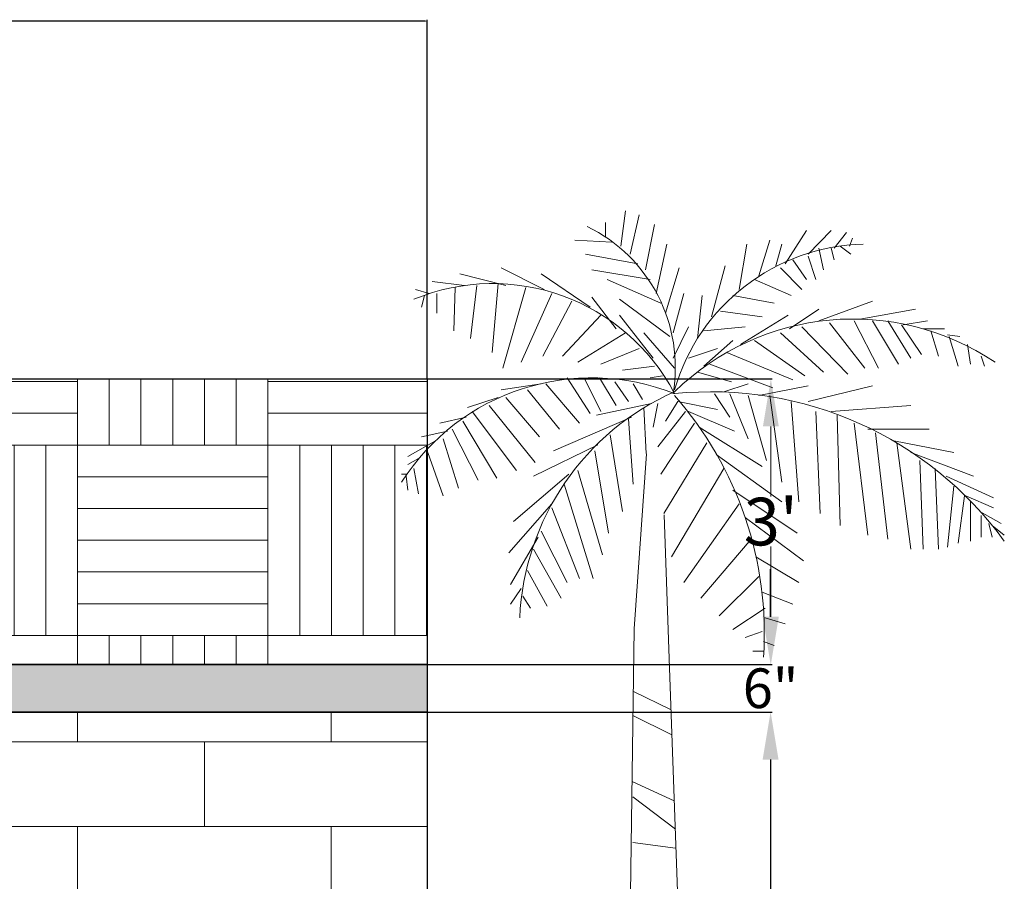
# Model space of a CAD drawing. Units: inches. Extents: x 37 to 824, y -700 to 234.
# Tile 21 of 77: x 377 to 501, y -487 to -378. Entities that reach past the tile are written whole.
import ezdxf

# ---------------------------------------------------------------- set-up
doc = ezdxf.new("R2010")
doc.units = ezdxf.units.IN
doc.header["$MEASUREMENT"] = 0
for name, color, linetype, lineweight in [('A-ANNO-DIMS', 2, 'Continuous', 18), ('A-ELEV', 3, 'Continuous', 25), ('A-ELEV-PATT', 8, 'Continuous', 13), ('A-SITE-PLNT', 3, 'Continuous', 13)]:
    doc.layers.add(name, color=color, linetype=linetype, lineweight=lineweight)
doc.styles.get("Standard").update_dxf_attribs({"font": 'arial.ttf'})
doc.dimstyles.get("Standard").update_dxf_attribs({"dimtxt": 0.18, "dimasz": 0.18, "dimexe": 0.18, "dimexo": 0.0625, "dimgap": 0.09, "dimtad": 0, "dimtih": 1, "dimtoh": 1, "dimdec": 1, "dimzin": 0, "dimdsep": 46, "dimlunit": 4, "dimtxsty": 'Standard', "dimcen": 0.09, "dimadec": 0, "dimazin": 0, "dimtfac": 1, "dimtdec": 1, "dimtofl": 0, "dimtmove": 0, "dimatfit": 3, "dimfxl": 1, "dimtolj": 1, "dimtzin": 0, "dimarcsym": 0})

# ---------------------------------------------------------------- blocks, each defined once
blk = doc.blocks.new('*D27')
at = {"layer": 'A-ANNO-DIMS', "color": 0, "lineweight": -2, "ltscale": 0.5, "transparency": 16777216}
for p, q in [((428.14, -465.63), (471.55, -465.63)), ((471.37, -471.63), (471.37, -522.47)), ((471.37, -579.63), (471.37, -528.78)), ((428.14, -585.63), (471.55, -585.63))]:
    blk.add_line(p, q, dxfattribs=at)
at = {"layer": 'A-ANNO-DIMS', "color": 0, "ltscale": 0.5, "transparency": 16777216}
for points in [[(470.37, -471.63), (472.37, -471.63), (471.37, -465.63)], [(470.37, -579.63), (472.37, -579.63), (471.37, -585.63)]]:
    blk.add_solid(points, dxfattribs=at)
at = {"layer": 'Defpoints', "color": 0, "ltscale": 0.5, "transparency": 16777216}
for p in [(428.08, -465.63), (471.37, -465.63), (428.08, -585.63)]:
    blk.add_point(p, dxfattribs=at)
at = {"layer": 'A-ANNO-DIMS', "color": 0, "ltscale": 0.5, "transparency": 16777216, "insert": (471.37, -525.63), "char_height": 6, "attachment_point": 5}
blk.add_mtext("\\A1;10'", dxfattribs=at)
blk = doc.blocks.new('*D29')
at = {"layer": 'A-ANNO-DIMS', "color": 0, "lineweight": -2, "ltscale": 0.5, "transparency": 16777216}
for p, q in [((471.38, -453.63), (471.38, -447.63)), ((428.14, -459.63), (471.56, -459.63)), ((428.14, -465.63), (471.56, -465.63)), ((471.38, -471.63), (471.38, -477.63))]:
    blk.add_line(p, q, dxfattribs=at)
at = {"layer": 'A-ANNO-DIMS', "color": 0, "ltscale": 0.5, "transparency": 16777216}
for points in [[(470.38, -453.63), (472.38, -453.63), (471.38, -459.63)], [(470.38, -471.63), (472.38, -471.63), (471.38, -465.63)]]:
    blk.add_solid(points, dxfattribs=at)
at = {"layer": 'Defpoints', "color": 0, "ltscale": 0.5, "transparency": 16777216}
for p in [(428.08, -459.63), (471.38, -459.63), (428.08, -465.63)]:
    blk.add_point(p, dxfattribs=at)
at = {"layer": 'A-ANNO-DIMS', "color": 0, "ltscale": 0.5, "transparency": 16777216, "insert": (471.38, -462.63), "char_height": 5, "attachment_point": 5}
blk.add_mtext('\\A1;6"', dxfattribs=at)
blk = doc.blocks.new('*D30')
at = {"layer": 'A-ANNO-DIMS', "color": 0, "lineweight": -2, "ltscale": 0.5, "transparency": 16777216}
for p, q in [((428.14, -423.63), (471.59, -423.63)), ((428.14, -459.63), (471.59, -459.63))]:
    blk.add_line(p, q, dxfattribs=at)
at = {"layer": 'A-ANNO-DIMS', "color": 0, "lineweight": 0, "ltscale": 0.5, "transparency": 16777216}
for p, q in [((471.41, -429.63), (471.41, -438.47)), ((471.41, -453.63), (471.41, -444.78))]:
    blk.add_line(p, q, dxfattribs=at)
at = {"layer": 'A-ANNO-DIMS', "color": 0, "ltscale": 0.5, "transparency": 16777216}
for points in [[(470.41, -429.63), (472.41, -429.63), (471.41, -423.63)], [(470.41, -453.63), (472.41, -453.63), (471.41, -459.63)]]:
    blk.add_solid(points, dxfattribs=at)
at = {"layer": 'Defpoints', "color": 0, "ltscale": 0.5, "transparency": 16777216}
for p in [(428.08, -423.63), (428.08, -459.63), (471.41, -459.63)]:
    blk.add_point(p, dxfattribs=at)
at = {"layer": 'A-ANNO-DIMS', "color": 0, "ltscale": 0.5, "transparency": 16777216, "insert": (471.41, -441.63), "char_height": 6, "attachment_point": 5}
blk.add_mtext("\\A1;3'", dxfattribs=at)
blk = doc.blocks.new('*U34')
for p, q in [((-5.567, 196.707), (-4.987, 201.167)), ((-4.407, 195.716), (-3.247, 200.672)), ((-7.5, 199.68), (-7.5, 197.946)), ((-2.474, 193.733), (-1.315, 199.433)), ((15.116, 194.477), (17.822, 198.689)), ((18.015, 195.716), (20.914, 198.689)), ((-6.727, 197.202), (-11.366, 197.45)), ((11.829, 192.99), (13.182, 197.45)), ((21.301, 196.459), (22.847, 198.441)), ((23.234, 196.707), (23.62, 197.698)), ((-1.121, 190.759), (0.232, 196.955)), ((9.317, 191.255), (10.283, 196.955)), ((13.956, 194.229), (14.729, 196.955)), ((19.368, 196.459), (19.948, 193.733)), ((20.914, 196.459), (21.301, 194.972)), ((22.074, 196.707), (23.427, 195.716)), ((-3.441, 194.477), (-10.013, 195.716)), ((16.082, 194.972), (17.822, 192.494)), ((18.015, 195.468), (18.981, 192.494)), ((-15.232, 191.255), (-20.644, 193.981)), ((-1.894, 192.494), (-9.24, 193.733)), ((0.038, 188.281), (1.778, 193.981)), ((5.837, 187.786), (7.577, 194.229)), ((14.536, 193.981), (17.242, 191.255)), ((-20.064, 191.751), (-25.863, 193.238)), ((-9.433, 189.025), (-15.618, 193.238)), ((-0.541, 189.52), (-7.307, 192.494)), ((11.25, 192.494), (15.889, 190.512)), ((-29.729, 190.759), (-31.469, 191.255)), ((-25.283, 191.751), (-29.342, 192.246)), ((-26.443, 191.503), (-26.636, 186.051)), ((-23.737, 191.751), (-24.51, 185.06)), ((-21.031, 191.998), (-21.804, 183.325)), ((-17.551, 191.503), (-20.451, 181.343)), ((-30.309, 190.512), (-30.695, 189.025)), ((-28.763, 190.759), (-28.763, 188.281)), ((-14.265, 190.759), (-18.131, 182.086)), ((-6.147, 186.299), (-9.24, 190.264)), ((-5.76, 190.016), (0.618, 185.308)), ((1.005, 185.803), (2.358, 190.759)), ((4.098, 185.06), (4.678, 190.512)), ((8.544, 190.512), (13.763, 189.52)), ((-11.753, 189.768), (-15.425, 182.83)), ((15.695, 186.299), (19.368, 188.777)), ((19.368, 187.29), (26.133, 189.768)), ((24.78, 187.538), (31.546, 188.777)), ((-8.08, 188.034), (-12.912, 182.83)), ((-5.76, 188.034), (-1.508, 182.582)), ((6.997, 188.529), (12.216, 187.786)), ((9.51, 184.317), (15.502, 188.034)), ((1.005, 182.582), (2.938, 186.547)), ((4.871, 186.051), (10.09, 186.547)), ((17.242, 186.547), (23.041, 180.599)), ((20.721, 187.042), (25.167, 181.343)), ((23.814, 187.29), (26.907, 181.343)), ((26.133, 187.29), (29.419, 181.838)), ((28.066, 187.29), (30.966, 182.582)), ((29.806, 186.795), (32.319, 183.078)), ((29.999, 186.795), (33.092, 187.29)), ((32.512, 186.299), (35.218, 186.299)), ((-4.987, 185.803), (-10.979, 182.086)), ((-2.668, 185.803), (1.198, 181.343)), ((14.536, 185.803), (19.948, 180.847)), ((33.479, 186.051), (34.445, 182.83)), ((35.605, 185.556), (37.151, 185.308)), ((35.798, 185.308), (36.958, 181.591)), ((-3.247, 183.821), (-8.08, 181.838)), ((2.938, 182.582), (6.61, 183.821)), ((4.871, 181.591), (8.544, 184.812)), ((11.25, 184.812), (17.628, 180.352)), ((38.118, 184.317), (38.504, 181.838)), ((7.77, 183.325), (16.082, 179.856)), ((39.857, 182.83), (40.244, 181.591)), ((-1.315, 181.591), (-5.374, 181.095)), ((5.644, 181.838), (13.569, 178.865)), ((-12.332, 180.104), (-9.433, 175.643)), ((-10.206, 180.104), (-8.08, 175.891)), ((-8.273, 180.104), (-6.147, 176.635)), ((-0.348, 180.352), (-1.894, 180.104)), ((4.098, 180.847), (8.35, 179.608)), ((-15.618, 179.36), (-20.644, 178.617)), ((-15.038, 179.36), (-10.786, 174.404)), ((-6.34, 179.608), (-4.6, 177.13)), ((-4.021, 179.36), (-2.861, 177.378)), ((7.384, 178.369), (10.476, 179.36)), ((11.829, 177.874), (18.015, 179.113)), ((18.015, 177.13), (26.133, 179.113)), ((-21.031, 177.626), (-24.897, 176.387)), ((-20.064, 177.626), (-15.812, 172.67)), ((-17.358, 178.617), (-13.299, 173.661)), ((6.224, 178.121), (8.157, 175.148)), ((8.157, 178.121), (10.476, 172.422)), ((10.476, 177.874), (12.796, 169.696)), ((13.182, 177.874), (14.729, 166.97)), ((-22.191, 176.635), (-16.391, 169.448)), ((-1.701, 176.882), (-8.66, 175.396)), ((-2.668, 176.387), (-2.376, 170.594)), ((-0.928, 176.882), (-1.508, 173.909)), ((1.585, 177.13), (0.038, 174.652)), ((1.585, 177.13), (6.61, 176.139)), ((15.889, 177.13), (16.855, 164.492)), ((20.914, 175.891), (30.966, 176.635)), ((-25.09, 175.148), (-28.376, 174.404)), ((-24.317, 175.891), (-18.711, 168.457)), ((-4.214, 175.148), (-14.072, 170.935)), ((2.551, 175.891), (-0.928, 171.431)), ((2.938, 175.891), (8.737, 173.413)), ((18.981, 175.891), (19.561, 163.005)), ((21.688, 175.396), (22.074, 161.518)), ((-25.476, 174.652), (-21.224, 167.466)), ((-4.6, 174.9), (-4.021, 166.722)), ((3.711, 174.404), (-0.541, 167.961)), ((4.291, 173.909), (12.216, 168.953)), ((23.814, 174.404), (25.554, 160.279)), ((-27.409, 173.413), (-30.695, 172.67)), ((-26.829, 173.661), (-23.544, 167.218)), ((-6.92, 172.917), (-5.374, 163.253)), ((25.554, 173.661), (33.285, 173.661)), ((26.52, 173.165), (28.066, 159.784)), ((-28.956, 172.174), (-32.435, 170.192)), ((-27.989, 172.422), (-26.056, 166.227)), ((-8.466, 171.678), (-16.585, 167.713)), ((5.257, 171.926), (-0.155, 163.005)), ((28.839, 172.174), (36.378, 170.687)), ((29.226, 171.926), (30.966, 158.545)), ((-29.922, 170.687), (-27.989, 165.235)), ((-8.853, 170.935), (-7.113, 160.527)), ((6.417, 170.439), (14.729, 164.492)), ((30.966, 170.687), (38.891, 167.713)), ((-31.082, 169.944), (-32.435, 169.2)), ((32.126, 169.696), (32.512, 158.545)), ((-32.628, 167.961), (-33.208, 167.961)), ((-32.628, 167.713), (-32.435, 165.979)), ((-31.662, 168.705), (-31.082, 165.483)), ((-12.139, 167.961), (-19.098, 162.014)), ((-10.979, 168.457), (-7.887, 157.801)), ((7.384, 168.705), (0.812, 157.553)), ((34.058, 168.705), (34.445, 158.545)), ((35.412, 167.713), (41.404, 164.988)), ((-12.719, 166.722), (-9.046, 154.828)), ((36.378, 166.474), (35.605, 158.792)), ((8.544, 165.979), (16.662, 160.527)), ((37.731, 165.235), (36.958, 159.288)), ((37.924, 165.235), (41.404, 163.749)), ((-14.265, 164.244), (-19.678, 158.049)), ((9.317, 164.244), (2.358, 154.332)), ((38.504, 164.492), (38.504, 159.536)), ((-14.265, 163.749), (-10.786, 154.828)), ((39.664, 163.253), (42.37, 161.766)), ((39.857, 162.757), (39.857, 160.031)), ((10.09, 162.51), (17.435, 157.058)), ((40.824, 161.766), (41.21, 160.031)), ((41.21, 161.518), (42.757, 160.279)), ((-15.618, 160.775), (-12.332, 154.332)), ((-16.005, 160.031), (-19.484, 154.084)), ((10.863, 159.784), (4.484, 152.35)), ((-16.585, 158.545), (-13.106, 152.35)), ((11.443, 157.553), (16.855, 154.332)), ((-17.358, 155.819), (-14.845, 151.358)), ((11.829, 155.075), (6.804, 150.119)), ((-18.131, 153.589), (-19.484, 151.606)), ((12.216, 153.093), (16.082, 151.606)), ((-17.938, 152.597), (-16.972, 151.111)), ((12.603, 151.111), (8.544, 148.385)), ((12.603, 149.872), (15.116, 149.128)), ((12.216, 148.137), (10.09, 147.393)), ((12.409, 146.898), (13.763, 146.402)), ((12.409, 145.659), (11.056, 145.659)), ((-4.081, 140.645), (0.753, 138.261)), ((-4.081, 137.547), (0.753, 135.163)), ((-4.081, 129.205), (1.124, 126.821)), ((-4.081, 127.298), (1.31, 123.246)), ((-4.081, 121.578), (1.31, 120.863))]:
    blk.add_line(p, q)
for points in [[(-2.363, 170.553), (-3.88, 148.505), (-4.988, 69.634), (-3.325, 24.869), (0, 0)], [(-0.116, 162.848), (0.554, 143.532), (2.217, 96.635), (3.88, 44.054), (7.76, 12.079), (11.64, 0)]]:
    blk.add_lwpolyline(points)
for centre, radius, start, end in [((-18.427, 181.448), 19.715, 350.285, 64.11229), ((25.595, 171.567), 25.395, 91.40319, 163.882), ((-21.738, 166.094), 25.899, 27.67115, 112.5305), ((23.687, 155.341), 32.188, 56.19272, 134.3213), ((-9.259, 151.732), 28.386, 68.38311, 147.5322), ((14.394, 148.393), 32.752, 113.7592, 177.4133), ((5.828, 132.718), 45.639, 35.98777, 95.82273), ((-32.8, 147.923), 45.309, 356.1943, 41.37848)]:
    blk.add_arc(centre, radius, start, end)
blk = doc.blocks.new('*D66')
at = {"layer": 'A-ANNO-DIMS', "color": 0, "lineweight": -2, "ltscale": 0.5, "transparency": 16777216}
for p, q in [((161.08, -423.56), (161.08, -378.38)), ((428.08, -423.56), (428.08, -378.38)), ((161.26, -378.56), (294.18, -378.56)), ((427.9, -378.56), (294.98, -378.56))]:
    blk.add_line(p, q, dxfattribs=at)
at = {"layer": 'A-ANNO-DIMS', "color": 0, "ltscale": 0.5, "transparency": 16777216}
for points in [[(161.26, -378.53), (161.26, -378.59), (161.08, -378.56)], [(427.9, -378.53), (427.9, -378.59), (428.08, -378.56)]]:
    blk.add_solid(points, dxfattribs=at)
at = {"layer": 'Defpoints', "color": 0, "ltscale": 0.5, "transparency": 16777216}
for p in [(428.08, -378.56), (161.08, -423.63), (428.08, -423.63)]:
    blk.add_point(p, dxfattribs=at)
at = {"layer": 'A-ANNO-DIMS', "color": 0, "ltscale": 0.5, "transparency": 16777216, "insert": (294.58, -378.56), "char_height": 0.18, "attachment_point": 5}
blk.add_mtext('\\A1;22\'-3"', dxfattribs=at)

msp = doc.modelspace()

# ---------------------------------------------------------------- hatches: boundary and pattern name
at = {"layer": 'A-ELEV-PATT', "ltscale": 0.5}
h = msp.add_hatch(dxfattribs=at)
h.set_pattern_fill('AR-PARQ1', color=256, scale=2)
h.paths.add_polyline_path([(428.08, -423.63), (161.08, -423.63), (161.08, -459.63), (428.08, -459.63)])
h = msp.add_hatch(color=256, dxfattribs=at)
h.dxf.hatch_style = 1
h.paths.add_polyline_path([(161.08, -459.63), (161.08, -465.63), (428.08, -465.63), (428.08, -459.63)])
h.paths.add_polyline_path([(229.03, -498.21), (214.53, -498.21), (214.53, -529.21), (229.03, -529.21)])
h.paths.add_polyline_path([(245.53, -498.21), (230.03, -498.21), (230.03, -529.21), (245.53, -529.21)])
h.paths.add_polyline_path([(315.2, -574.01), (341.2, -574.01), (341.2, -505.03), (315.2, -505.03)])
h = msp.add_hatch(dxfattribs=at)
h.set_pattern_fill('AR-BRSTD', color=256, scale=4)
h.paths.add_polyline_path([(299.08, -489.63), (358.13, -489.63), (358.13, -585.63), (428.08, -585.63), (428.08, -465.63), (161.08, -465.63), (161.08, -585.63), (299.08, -585.63)])
h.paths.add_polyline_path([(205.08, -537.63), (205.08, -489.63), (255.08, -489.63), (255.08, -537.63)], flags=16)

# ---------------------------------------------------------------- linework, layer by layer
at = {"layer": 'A-ELEV', "ltscale": 0.5}
for points in [[(161.08, -423.63), (428.08, -423.63), (428.08, -459.63), (161.08, -459.63)], [(161.08, -459.63), (428.08, -459.63), (428.08, -465.63), (161.08, -465.63)], [(161.08, -465.63), (428.08, -465.63), (428.08, -585.63), (161.08, -585.63)]]:
    msp.add_lwpolyline(points, close=True, dxfattribs=at)

# ---------------------------------------------------------------- block references
at = {"layer": 'A-SITE-PLNT'}
msp.add_blockref('*U34', (458.08, -603.63), dxfattribs=at)

# ---------------------------------------------------------------- dimensions: what is measured, and where the dimension line sits
at = {"layer": 'A-ANNO-DIMS', "ltscale": 0.5}
dim = msp.add_linear_dim(base=(428.08, -378.56), p1=(161.08, -423.63), p2=(428.08, -423.63), dimstyle='Standard', override={"dimdec": 1, "dimlfac": 1, "dimrnd": 0, "dimzin": 1, "dimdsep": 46, "dimlunit": 4, "dimfrac": 2}, dxfattribs=at)
dim.commit()
dim.dimension.update_dxf_attribs({"geometry": '*D66', "text_midpoint": (294.58, -378.56)})
for base, p1, p2, override, picture, middle in [((471.41, -459.63), (428.08, -423.63), (428.08, -459.63), {"dimtxt": 6, "dimasz": 6, "dimclrd": 0, "dimclre": 0, "dimclrt": 0, "dimlwd": 0}, '*D30', (471.41, -441.63)), ((471.38, -459.63), (428.08, -465.63), (428.08, -459.63), {"dimtxt": 5, "dimasz": 6, "dimclrd": 0, "dimclre": 0, "dimclrt": 0}, '*D29', (471.38, -462.63)), ((471.37, -465.63), (428.08, -585.63), (428.08, -465.63), {"dimtxt": 6, "dimasz": 6, "dimclrd": 0, "dimclre": 0, "dimclrt": 0}, '*D27', (471.37, -525.63))]:
    dim = msp.add_linear_dim(base=base, p1=p1, p2=p2, angle=90, dimstyle='Standard', override=override, dxfattribs=at)
    dim.commit()
    dim.dimension.update_dxf_attribs({"geometry": picture, "text_midpoint": middle})

doc.saveas('drawing.dxf')
